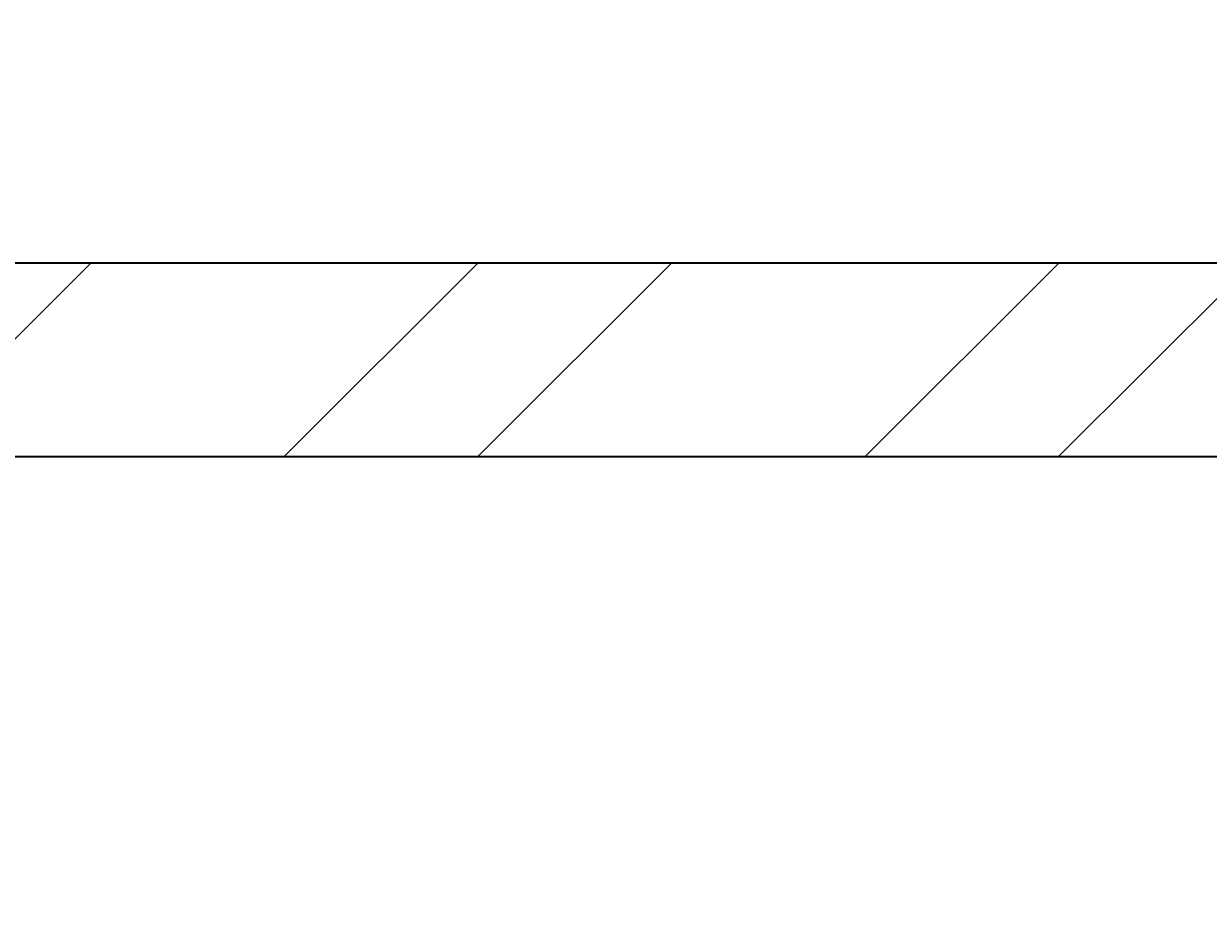
# Model space of a CAD drawing. Units: inches. Extents: x 1962 to 2771, y 1245 to 2660.
# Tile 68 of 114: x 2523 to 2551, y 2115 to 2135. Entities that reach past the tile are written whole.
import ezdxf

# ---------------------------------------------------------------- set-up
doc = ezdxf.new("R2010")
doc.units = ezdxf.units.IN
for name, color, linetype, lineweight in [('A-ANNO-DIMS', 2, 'Continuous', 18), ('A-WALL', 7, 'Continuous', 35), ('A-WALL-PATT', 252, 'Continuous', 13)]:
    doc.layers.add(name, color=color, linetype=linetype, lineweight=lineweight)
doc.styles.get("Standard").update_dxf_attribs({"font": 'arial.ttf'})
doc.dimstyles.get("Standard").update_dxf_attribs({"dimtxt": 0.18, "dimasz": 0.18, "dimexe": 0.18, "dimexo": 0.0625, "dimgap": 0.09, "dimtad": 0, "dimtih": 1, "dimtoh": 1, "dimdec": 4, "dimzin": 0, "dimdsep": 46, "dimtxsty": 'Standard', "dimcen": 0.09, "dimadec": 0, "dimazin": 0, "dimtfac": 1, "dimtdec": 4, "dimtofl": 0, "dimtmove": 0, "dimatfit": 3, "dimfxl": 1, "dimtolj": 1, "dimtzin": 0, "dimarcsym": 0})

# ---------------------------------------------------------------- blocks, each defined once
blk = doc.blocks.new('*D40')
at = {"layer": 'A-ANNO-DIMS', "color": 0, "lineweight": -2, "transparency": 16777216}
for p, q in [((2072.02, 2033.906), (2072.02, 2583.474)), ((2660.807, 2524.406), (2660.807, 2583.474)), ((2072.2, 2583.294), (2366.02, 2583.294)), ((2660.627, 2583.294), (2366.808, 2583.294))]:
    blk.add_line(p, q, dxfattribs=at)
at = {"layer": 'A-ANNO-DIMS', "color": 0, "transparency": 16777216}
for points in [[(2072.2, 2583.324), (2072.2, 2583.264), (2072.02, 2583.294)], [(2660.627, 2583.324), (2660.627, 2583.264), (2660.807, 2583.294)]]:
    blk.add_solid(points, dxfattribs=at)
at = {"layer": 'Defpoints', "color": 0, "transparency": 16777216}
for p in [(2660.807, 2583.294), (2660.807, 2524.344), (2072.02, 2033.844)]:
    blk.add_point(p, dxfattribs=at)
at = {"layer": 'A-ANNO-DIMS', "color": 0, "transparency": 16777216, "insert": (2366.414, 2583.294), "char_height": 0.18, "attachment_point": 5}
blk.add_mtext('\\A1;588.8', dxfattribs=at)

msp = doc.modelspace()

# ---------------------------------------------------------------- hatches: boundary and pattern name
at = {"layer": 'A-WALL-PATT'}
h = msp.add_hatch(dxfattribs=at)
h.set_pattern_fill('ANSI32', color=256)
h.paths.add_polyline_path([(2090.8074, 2467.3437), (2141.6481, 2467.3437), (2141.6481, 2469.5937), (2141.6481, 2471.8437), (2086.3074, 2471.8437), (2086.3074, 2422.5333), (2090.8074, 2422.5333)])
h.paths.add_polyline_path([(2282.7664, 2471.8437), (2204.8982, 2471.8437), (2204.8982, 2467.3437), (2234.8074, 2467.3437), (2234.8074, 2311.3437), (2228.7492, 2311.3437), (2228.7492, 2306.8437), (2234.8074, 2306.8437), (2331.9227, 2306.8437), (2331.9227, 2309.0937), (2331.9227, 2311.3437), (2239.3074, 2311.3437), (2239.3074, 2467.3437), (2282.7664, 2467.3437), (2282.7664, 2469.5937)])
h.paths.add_polyline_path([(2471.4531, 2519.8437), (2552.011, 2519.8437), (2564.3996, 2519.8437), (2564.3996, 2511.1389), (2568.8996, 2511.1389), (2568.8996, 2524.3437), (2466.9531, 2524.3437), (2466.9531, 2471.8437), (2450.0749, 2471.8437), (2446.4672, 2471.8437), (2446.4672, 2467.3437), (2450.0749, 2467.3437), (2475.9988, 2467.3437), (2475.9988, 2469.5937), (2475.9988, 2471.8437), (2471.4531, 2471.8437)])
h.paths.add_polyline_path([(2575.2231, 2469.5937), (2575.2231, 2471.8437), (2568.8996, 2471.8437), (2568.8996, 2487.1389), (2564.3996, 2487.1389), (2564.3996, 2471.8437), (2556.511, 2471.8437), (2499.2904, 2471.8437), (2499.2904, 2467.3437), (2507.8074, 2467.3437), (2507.8074, 2311.3437), (2414.863, 2311.3437), (2414.863, 2306.8437), (2512.3074, 2306.8437), (2517.0114, 2306.8437), (2517.0114, 2309.0937), (2517.0114, 2311.3437), (2512.3074, 2311.3437), (2512.3074, 2467.3437), (2575.2231, 2467.3437)])
h.paths.add_polyline_path([(2660.8074, 2471.8437), (2600.9602, 2471.8437), (2600.9602, 2467.3437), (2656.3074, 2467.3437), (2656.3074, 2432.5704), (2660.8074, 2432.5704)])
h.paths.add_polyline_path([(2660.8074, 2372.5704), (2656.3074, 2372.5704), (2656.3074, 2311.3437), (2600.276, 2311.3437), (2600.276, 2309.0937), (2600.276, 2306.8437), (2656.3074, 2306.8437), (2656.3074, 2296.2593), (2660.8074, 2296.2593)])
h.paths.add_polyline_path([(2572.3074, 2306.8437), (2577.1385, 2306.8437), (2577.1385, 2311.3437), (2551.082, 2311.3437), (2551.082, 2306.8437), (2567.8074, 2306.8437), (2567.8074, 2258.8437), (2540.0574, 2258.8437), (2540.0574, 2256.5937), (2540.0574, 2254.3437), (2567.8074, 2254.3437), (2656.3074, 2254.3437), (2656.3074, 2236.9085), (2660.8074, 2236.9085), (2660.8074, 2272.2593), (2656.3074, 2272.2593), (2656.3074, 2258.8437), (2572.3074, 2258.8437)])
h.paths.add_polyline_path([(2512.3074, 2254.3437), (2518.8716, 2254.3437), (2518.8716, 2256.5937), (2518.8716, 2258.8437), (2507.8074, 2258.8437), (2507.8074, 2177.8437), (2567.8074, 2177.8437), (2567.8074, 2172.9628), (2572.3074, 2172.9628), (2572.3074, 2177.8437), (2656.3074, 2177.8437), (2656.3074, 2166.4846), (2660.8074, 2166.4846), (2660.8074, 2200.9085), (2656.3074, 2200.9085), (2656.3074, 2182.3437), (2512.3074, 2182.3437)])
h.paths.add_polyline_path([(2656.3074, 2129.8437), (2572.3074, 2129.8437), (2572.3074, 2150.3044), (2570.0574, 2150.3044), (2567.8074, 2150.3044), (2567.8074, 2129.8437), (2507.8074, 2129.8437), (2507.8074, 2116.3027), (2510.0574, 2116.3027), (2512.3074, 2116.3027), (2512.3074, 2125.3437), (2567.8074, 2125.3437), (2572.3074, 2125.3437), (2656.3074, 2125.3437)])
h.paths.add_polyline_path([(2090.8074, 2362.5333), (2086.3074, 2362.5333), (2086.3074, 2298.6242), (2090.8074, 2298.6242), (2090.8074, 2306.8437), (2174.8074, 2306.8437), (2174.8074, 2286.4178), (2179.3074, 2286.4178), (2179.3074, 2306.8437), (2192.8641, 2306.8437), (2192.8641, 2309.0937), (2192.8641, 2311.3437), (2090.8074, 2311.3437)])
h.paths.add_polyline_path([(2209.156, 2258.8437), (2179.3074, 2258.8437), (2179.3074, 2263.2236), (2177.0574, 2263.2236), (2174.8074, 2263.2236), (2174.8074, 2258.8437), (2090.8074, 2258.8437), (2090.8074, 2274.6242), (2086.3074, 2274.6242), (2086.3074, 2238.2967), (2088.5574, 2238.2967), (2090.8074, 2238.2967), (2090.8074, 2254.3437), (2209.156, 2254.3437)])
h.paths.add_polyline_path([(2090.8074, 2177.8437), (2234.8074, 2177.8437), (2234.8074, 2173.1428), (2239.3074, 2173.1428), (2239.3074, 2258.8437), (2230.8442, 2258.8437), (2230.8442, 2256.5937), (2230.8442, 2254.3437), (2234.8074, 2254.3437), (2234.8074, 2182.3437), (2090.8074, 2182.3437), (2090.8074, 2202.2967), (2086.3074, 2202.2967), (2086.3074, 2140.0389), (2090.8074, 2140.0389)])
h.paths.add_polyline_path([(2090.8074, 2080.0389), (2086.3074, 2080.0389), (2086.3074, 2033.8437), (2090.8074, 2033.8437)], flags=17)
h.paths.add_polyline_path([(2244.9405, 2033.8437), (2239.3074, 2033.8437), (2239.3074, 2142.0665), (2237.2592, 2142.0665), (2234.8074, 2142.0665), (2234.8074, 2033.8437), (2090.8074, 2033.8437), (2076.5204, 2033.8437), (2072.0204, 2033.8437), (2072.0204, 2000.4493), (2076.5204, 2000.4493), (2076.5204, 2029.3437), (2090.8074, 2029.3437), (2244.9405, 2029.3437), (2244.9405, 2031.5937)])
h.paths.add_polyline_path([(2234.8074, 1933.3437), (2076.5204, 1933.3437), (2076.5204, 1952.4493), (2074.2704, 1952.4493), (2072.0204, 1952.4493), (2072.0204, 1933.3437), (2072.0204, 1928.8437), (2234.8074, 1928.8437)])
h.paths.add_polyline_path([(2090.8074, 1928.8437), (2086.3074, 1928.8437), (2086.3074, 1906.5013), (2090.8074, 1906.5013)])
h.paths.add_polyline_path([(2090.8074, 1846.5013), (2086.3074, 1846.5013), (2086.3074, 1769.9917), (2088.5574, 1769.9917), (2090.8074, 1769.9917), (2090.8074, 1780.3437), (2234.8074, 1780.3437), (2234.8074, 1708.3437), (2230.3764, 1708.3437), (2230.3764, 1703.8437), (2239.3074, 1703.8437), (2239.3074, 1792.6669), (2237.0574, 1792.6669), (2234.8074, 1792.6669), (2234.8074, 1784.8437), (2090.8074, 1784.8437)])
h.paths.add_polyline_path([(2239.3074, 1928.8437), (2244.9405, 1928.8437), (2244.9405, 1931.0937), (2244.9405, 1933.3437), (2234.8074, 1933.3437), (2234.8074, 1928.8437), (2234.8074, 1825.5949), (2239.3074, 1825.5949)])
h.paths.add_polyline_path([(2148.0425, 1649.0937), (2148.0425, 1651.3437), (2090.8074, 1651.3437), (2090.8074, 1646.8437), (2148.0425, 1646.8437)], flags=0)
h.paths.add_polyline_path([(2207.5601, 1708.3437), (2090.8074, 1708.3437), (2090.8074, 1703.8437), (2174.8074, 1703.8437), (2174.8074, 1651.3437), (2170.4457, 1651.3437), (2170.4457, 1646.8437), (2195.9924, 1646.8437), (2195.9924, 1649.0937), (2195.9924, 1651.3437), (2179.3074, 1651.3437), (2179.3074, 1703.8437), (2207.5601, 1703.8437), (2207.5601, 1706.0937)])
h.paths.add_polyline_path([(2090.8074, 1733.9917), (2086.3074, 1733.9917), (2086.3074, 1696.1032), (2088.5574, 1696.1032), (2090.8074, 1696.1032)])
h.paths.add_polyline_path([(2090.8074, 1672.1032), (2086.3074, 1672.1032), (2086.3074, 1600.3335), (2090.8074, 1600.3335)])
h.paths.add_polyline_path([(2090.8074, 1540.3335), (2086.3074, 1540.3335), (2086.3074, 1486.3437), (2139.6766, 1486.3437), (2139.6766, 1490.8437), (2090.8074, 1490.8437)])
h.paths.add_polyline_path([(2302.3876, 1490.8437), (2239.3074, 1490.8437), (2239.3074, 1646.8437), (2335.9994, 1646.8437), (2335.9994, 1651.3437), (2229.884, 1651.3437), (2229.884, 1646.8437), (2234.8074, 1646.8437), (2234.8074, 1490.8437), (2202.7103, 1490.8437), (2202.7103, 1488.5937), (2202.7103, 1486.3437), (2275.0699, 1486.3437), (2275.0699, 1475.772), (2279.5699, 1475.772), (2279.5699, 1486.3437), (2302.3876, 1486.3437)])
h.paths.add_polyline_path([(2279.5699, 1451.772), (2275.0699, 1451.772), (2275.0699, 1438.3437), (2174.8074, 1438.3437), (2174.8074, 1486.3437), (2179.7922, 1486.3437), (2179.7922, 1490.8437), (2163.3585, 1490.8437), (2163.3585, 1488.5937), (2163.3585, 1486.3437), (2170.3074, 1486.3437), (2170.3074, 1433.8437), (2279.5699, 1433.8437)])
h.paths.add_polyline_path([(2427.2363, 1490.8437), (2375.8074, 1490.8437), (2375.8074, 1646.8437), (2381.6401, 1646.8437), (2381.6401, 1651.3437), (2365.887, 1651.3437), (2365.887, 1649.0937), (2365.887, 1646.8437), (2371.3074, 1646.8437), (2371.3074, 1490.8437), (2327.5627, 1490.8437), (2327.5627, 1488.5937), (2327.5627, 1486.3437), (2371.3074, 1486.3437), (2371.3074, 1433.8437), (2375.8074, 1433.8437), (2375.8074, 1486.3437), (2427.2363, 1486.3437)])
h.paths.add_polyline_path([(2512.3074, 1646.8437), (2519.4351, 1646.8437), (2519.4351, 1649.0937), (2519.4351, 1651.3437), (2507.8074, 1651.3437), (2416.0063, 1651.3437), (2416.0063, 1649.0937), (2416.0063, 1646.8437), (2507.8074, 1646.8437), (2507.8074, 1490.8437), (2497.0532, 1490.8437), (2497.0532, 1488.5937), (2497.0532, 1486.3437), (2574.9344, 1486.3437), (2574.9344, 1476.0181), (2579.4344, 1476.0181), (2579.4344, 1486.3437), (2584.4872, 1486.3437), (2584.3074, 1490.8437), (2512.3074, 1490.8437)])
h.paths.add_polyline_path([(2470.5091, 1486.3437), (2473.9767, 1486.3437), (2473.9767, 1490.8437), (2449.6605, 1490.8437), (2449.6605, 1488.5937), (2449.6605, 1486.3437), (2466.0091, 1486.3437), (2466.0091, 1433.8437), (2470.5091, 1433.8437), (2579.4344, 1433.8437), (2579.4344, 1452.0181), (2574.9344, 1452.0181), (2574.9344, 1438.3437), (2554.5091, 1438.3437), (2470.5091, 1438.3437)])
h.paths.add_polyline_path([(2656.3074, 1490.8437), (2611.86, 1490.8437), (2611.86, 1486.3437), (2656.3074, 1486.3437)])
h.paths.add_polyline_path([(2660.8074, 1532.7007), (2658.5574, 1532.7007), (2656.3074, 1532.7007), (2656.3074, 1486.3437), (2660.8074, 1486.3437)])
h.paths.add_polyline_path([(2660.8074, 1664.9663), (2656.3074, 1664.9663), (2656.3074, 1651.3437), (2602.2313, 1651.3437), (2602.2313, 1646.8437), (2656.3074, 1646.8437), (2656.3074, 1592.7007), (2660.8074, 1592.7007)])
h.paths.add_polyline_path([(2660.8074, 1724.5221), (2656.3074, 1724.5221), (2656.3074, 1703.8437), (2542.4725, 1703.8437), (2542.4725, 1699.3437), (2567.8074, 1699.3437), (2567.8074, 1651.3437), (2552.7766, 1651.3437), (2552.7766, 1649.0937), (2552.7766, 1646.8437), (2577.2878, 1646.8437), (2577.2878, 1649.0937), (2577.2878, 1651.3437), (2572.3074, 1651.3437), (2572.3074, 1699.3437), (2656.3074, 1699.3437), (2656.3074, 1688.9663), (2660.8074, 1688.9663)])
h.paths.add_polyline_path([(2660.8074, 1880.6524), (2656.3074, 1880.6524), (2656.3074, 1832.8437), (2512.3074, 1832.8437), (2512.3074, 1837.8959), (2507.8074, 1837.8959), (2507.8074, 1828.3437), (2567.8074, 1828.3437), (2567.8074, 1804.3437), (2572.3074, 1804.3437), (2572.3074, 1828.3437), (2656.3074, 1828.3437), (2656.3074, 1818.6778), (2660.8074, 1818.6778)])
h.paths.add_polyline_path([(2660.8074, 1794.6778), (2656.3074, 1794.6778), (2656.3074, 1780.3437), (2572.3074, 1780.3437), (2572.3074, 1783.0303), (2570.0574, 1783.0303), (2567.8074, 1783.0303), (2567.8074, 1780.3437), (2507.8074, 1780.3437), (2507.8074, 1699.3437), (2517.8858, 1699.3437), (2517.8858, 1701.5937), (2517.8858, 1703.8437), (2512.3074, 1703.8437), (2512.3074, 1775.8437), (2656.3074, 1775.8437), (2656.3074, 1760.5221), (2660.8074, 1760.5221)])
h.paths.add_polyline_path([(2660.8074, 1981.3437), (2660.8074, 2020.2808), (2658.5574, 2020.2808), (2656.3074, 2020.2808), (2656.3074, 1981.3437), (2512.3074, 1981.3437), (2512.3074, 2086.6996), (2507.8074, 2086.6996), (2507.8074, 1981.3437), (2375.8074, 1981.3437), (2375.8074, 1986.8505), (2373.5574, 1986.8505), (2371.3074, 1986.8505), (2371.3074, 1973.2607), (2375.8074, 1973.2607), (2375.8074, 1976.8437), (2507.8074, 1976.8437), (2507.8074, 1865.4281), (2510.0574, 1865.4281), (2512.3074, 1865.4281), (2512.3074, 1976.8437), (2660.8074, 1976.8437)])
h.paths.add_polyline_path([(2375.8074, 1940.297), (2373.5574, 1940.297), (2371.3074, 1940.297), (2371.3074, 1933.3437), (2278.4434, 1933.3437), (2278.4434, 1928.8437), (2371.3074, 1928.8437), (2371.3074, 1651.3437), (2375.8074, 1651.3437)])
h.paths.add_polyline_path([(2660.8074, 1976.8437), (2656.3074, 1976.8437), (2656.3074, 1940.6524), (2660.8074, 1940.6524)], flags=17)
h.paths.add_polyline_path([(2660.8074, 2142.4846), (2656.3074, 2142.4846), (2656.3074, 2080.2808), (2660.8074, 2080.2808)])
h.paths.add_polyline_path([(2381.4189, 2311.3437), (2375.8074, 2311.3437), (2375.8074, 2467.3437), (2424.7242, 2467.3437), (2424.7242, 2469.5937), (2424.7242, 2471.8437), (2375.8074, 2471.8437), (2375.8074, 2524.3437), (2371.3074, 2524.3437), (2371.3074, 2471.8437), (2307.2097, 2471.8437), (2307.2097, 2467.3437), (2371.3074, 2467.3437), (2371.3074, 2311.3437), (2366.8901, 2311.3437), (2366.8901, 2306.8437), (2371.3074, 2306.8437), (2371.3074, 2033.8437), (2279.6589, 2033.8437), (2279.6589, 2029.3437), (2371.3074, 2029.3437), (2371.3074, 2014.2598), (2375.8074, 2014.2598), (2375.8074, 2306.8437), (2381.4189, 2306.8437)])
h.paths.add_polyline_path([(2263.3074, 2524.3437), (2170.3074, 2524.3437), (2170.3074, 2519.8437), (2170.3074, 2471.8437), (2165.0312, 2471.8437), (2165.0312, 2467.3437), (2179.6721, 2467.3437), (2179.6721, 2469.5161), (2179.6721, 2471.8437), (2174.8074, 2471.8437), (2174.8074, 2519.8437), (2258.8074, 2519.8437), (2258.8074, 2511.6436), (2263.3074, 2511.6436)])
h.paths.add_polyline_path([(2245.0232, 1361.4123), (2492.9468, 1361.4123), (2492.9468, 1398.505), (2245.0232, 1398.505)], flags=9)
h.paths.add_polyline_path([(2388.1434, 2086.6936), (2425.0704, 2086.6936), (2425.0704, 2105.3509), (2388.1434, 2105.3509)], flags=9)
h.paths.add_polyline_path([(2404.922, 2242.6744), (2445.7337, 2242.6744), (2445.7337, 2261.3318), (2404.922, 2261.3318)], flags=9)
h.paths.add_polyline_path([(2269.4107, 2156.7935), (2306.3378, 2156.7935), (2306.3378, 2175.4508), (2269.4107, 2175.4508)], flags=9)
h.paths.add_polyline_path([(2269.3277, 2233.4343), (2306.2547, 2233.4343), (2306.2547, 2252.0917), (2269.3277, 2252.0917)], flags=9)
h.paths.add_polyline_path([(2431.6052, 2320.6922), (2470.4456, 2320.6922), (2470.4456, 2339.3495), (2431.6052, 2339.3495)], flags=25)
h.paths.add_polyline_path([(2249.6902, 2315.7608), (2288.5306, 2315.7608), (2288.5306, 2334.4182), (2249.6902, 2334.4182)], flags=25)
h.paths.add_polyline_path([(2096.9301, 2314.3181), (2135.7704, 2314.3181), (2135.7704, 2332.9755), (2096.9301, 2332.9755)], flags=25)
h.paths.add_polyline_path([(2134.3475, 2285.7089), (2161.4655, 2285.7089), (2161.4655, 2304.3662), (2134.3475, 2304.3662)], flags=9)
h.paths.add_polyline_path([(2126.5155, 2209.4076), (2159.9227, 2209.4076), (2159.9227, 2228.065), (2126.5155, 2228.065)], flags=25)
h.paths.add_polyline_path([(2110.5753, 2141.5299), (2149.4157, 2141.5299), (2149.4157, 2160.1872), (2110.5753, 2160.1872)], flags=25)
h.paths.add_polyline_path([(2249.8618, 1968.3317), (2286.3966, 1968.3317), (2286.3966, 1986.989), (2249.8618, 1986.989)], flags=9)
h.paths.add_polyline_path([(2395.9507, 1777.0051), (2436.7624, 1777.0051), (2436.7624, 1795.6625), (2395.9507, 1795.6625)], flags=9)
h.paths.add_polyline_path([(2398.5259, 1888.5651), (2435.0062, 1888.5651), (2435.0062, 1907.2224), (2398.5259, 1907.2224)], flags=25)
h.paths.add_polyline_path([(2259.3506, 1728.3559), (2296.2776, 1728.3559), (2296.2776, 1747.0132), (2259.3506, 1747.0132)], flags=9)
h.paths.add_polyline_path([(2271.3698, 1845.268), (2308.2968, 1845.268), (2308.2968, 1863.9253), (2271.3698, 1863.9253)], flags=9)
h.paths.add_polyline_path([(2120.9355, 1786.3027), (2159.7759, 1786.3027), (2159.7759, 1804.9601), (2120.9355, 1804.9601)], flags=25)
h.paths.add_polyline_path([(2121.3164, 1732.1043), (2154.7236, 1732.1043), (2154.7236, 1750.7616), (2121.3164, 1750.7616)], flags=25)
h.paths.add_polyline_path([(2118.3706, 1678.8997), (2147.5282, 1678.8997), (2147.5282, 1697.557), (2118.3706, 1697.557)], flags=25)
h.paths.add_polyline_path([(2385.9227, 1493.557), (2424.763, 1493.557), (2424.763, 1512.2143), (2385.9227, 1512.2143)], flags=25)
h.paths.add_polyline_path([(2248.7058, 1500.0256), (2287.5462, 1500.0256), (2287.5462, 1518.6829), (2248.7058, 1518.6829)], flags=25)
h.paths.add_polyline_path([(2104.1669, 1617.3771), (2143.0073, 1617.3771), (2143.0073, 1636.0344), (2104.1669, 1636.0344)], flags=9)
h.paths.add_polyline_path([(2096.0714, 1447.8824), (2137.3845, 1447.8824), (2137.3845, 1458.1859), (2096.0714, 1458.1859)], flags=9)
h.paths.add_polyline_path([(2180.6114, 1440.325), (2209.7689, 1440.325), (2209.7689, 1458.9823), (2180.6114, 1458.9823)], flags=25)
h.paths.add_polyline_path([(2316.1698, 1447.9637), (2357.4829, 1447.9637), (2357.4829, 1458.2673), (2316.1698, 1458.2673)], flags=9)
h.paths.add_polyline_path([(2397.6187, 1447.9637), (2438.9318, 1447.9637), (2438.9318, 1458.2673), (2397.6187, 1458.2673)], flags=9)
h.paths.add_polyline_path([(2473.0778, 1439.5953), (2502.2354, 1439.5953), (2502.2354, 1458.2527), (2473.0778, 1458.2527)], flags=25)
h.paths.add_polyline_path([(2589.7027, 1447.8819), (2631.0158, 1447.8819), (2631.0158, 1458.1855), (2589.7027, 1458.1855)], flags=9)
h.paths.add_polyline_path([(2522.4009, 1497.5285), (2561.2413, 1497.5285), (2561.2413, 1516.1859), (2522.4009, 1516.1859)], flags=25)
h.paths.add_polyline_path([(2579.6565, 1671.3482), (2608.8141, 1671.3482), (2608.8141, 1690.0056), (2579.6565, 1690.0056)], flags=25)
h.paths.add_polyline_path([(2544.7038, 1725.5064), (2578.1111, 1725.5064), (2578.1111, 1744.1637), (2544.7038, 1744.1637)], flags=25)
h.paths.add_polyline_path([(2578.1191, 1807.472), (2607.2766, 1807.472), (2607.2766, 1826.1293), (2578.1191, 1826.1293)], flags=25)
h.paths.add_polyline_path([(2595.0614, 1835.1839), (2633.9018, 1835.1839), (2633.9018, 1853.8413), (2595.0614, 1853.8413)], flags=25)
h.paths.add_polyline_path([(2567.0097, 2097.7035), (2605.8501, 2097.7035), (2605.8501, 2116.3609), (2567.0097, 2116.3609)], flags=9)
h.paths.add_polyline_path([(2586.644, 2134.6454), (2615.8015, 2134.6454), (2615.8015, 2153.3027), (2586.644, 2153.3027)], flags=9)
h.paths.add_polyline_path([(2544.6185, 2212.6783), (2578.0258, 2212.6783), (2578.0258, 2231.3356), (2544.6185, 2231.3356)], flags=25)
h.paths.add_polyline_path([(2577.0273, 2256.9023), (2606.1849, 2256.9023), (2606.1849, 2275.5597), (2577.0273, 2275.5597)], flags=24)
h.paths.add_polyline_path([(2605.2683, 2315.2821), (2644.1087, 2315.2821), (2644.1087, 2333.9395), (2605.2683, 2333.9395)], flags=25)
h.paths.add_polyline_path([(2583.1244, 2496.1815), (2624.4375, 2496.1815), (2624.4375, 2506.4851), (2583.1244, 2506.4851)], flags=9)
h.paths.add_polyline_path([(2474.761, 2497.0823), (2503.9185, 2497.0823), (2503.9185, 2515.7397), (2474.761, 2515.7397)], flags=25)
h.paths.add_polyline_path([(2387.5787, 2494.2563), (2428.902, 2494.2563), (2428.902, 2504.5598), (2387.5787, 2504.5598)], flags=9)
h.paths.add_polyline_path([(2300.1657, 2500.1564), (2341.4788, 2500.1564), (2341.4788, 2510.46), (2300.1657, 2510.46)], flags=25)
h.paths.add_polyline_path([(2176.8589, 2497.5843), (2206.0165, 2497.5843), (2206.0165, 2516.2416), (2176.8589, 2516.2416)], flags=25)
h.paths.add_polyline_path([(2097.4668, 2494.9762), (2138.7799, 2494.9762), (2138.7799, 2505.2798), (2097.4668, 2505.2798)], flags=9)

# ---------------------------------------------------------------- linework, layer by layer
at = {"layer": 'A-WALL'}
for p, q in [((2567.8074, 2129.8437), (2507.8074, 2129.8437)), ((2567.8074, 2125.3437), (2512.3074, 2125.3437))]:
    msp.add_line(p, q, dxfattribs=at)

# ---------------------------------------------------------------- dimensions: what is measured, and where the dimension line sits
at = {"layer": 'A-ANNO-DIMS'}
dim = msp.add_linear_dim(base=(2660.8074, 2583.2937), p1=(2072.0204, 2033.8437), p2=(2660.8074, 2524.3437), dimstyle='Standard', override={"dimdec": 1, "dimlfac": 1, "dimrnd": 0, "dimzin": 0, "dimdsep": 46, "dimlunit": 2}, dxfattribs=at)
dim.commit()
dim.dimension.update_dxf_attribs({"geometry": '*D40', "text_midpoint": (2366.4139, 2583.2937)})

doc.saveas('drawing.dxf')
